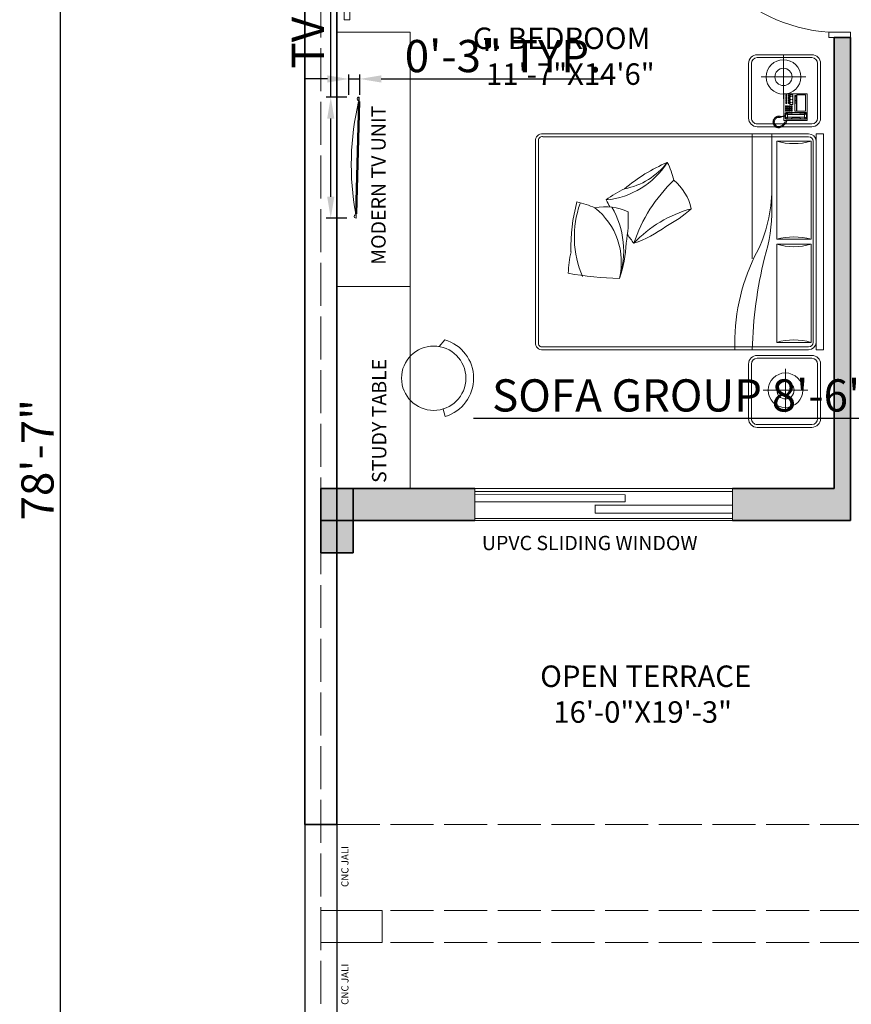
# Model space of a CAD drawing. Units: millimetres. Extents: x 595116 to 630915, y 909473 to 920225.
# Tile 129 of 134: x 630214 to 630446, y 919466 to 919741. Entities that reach past the tile are written whole.
import ezdxf

# ---------------------------------------------------------------- set-up
doc = ezdxf.new("R2010")
doc.units = ezdxf.units.MM
doc.linetypes.add('ACAD_ISO02W100', pattern=[15, 12, -3])
for name, color, linetype, lineweight in [('A-AREA-IDEN', 7, 'Continuous', 20), ('A-EQPM', 8, 'Continuous', 13), ('A-FLOR-SCRN', 31, 'Continuous', 18), ('A-FLOR-SCRN-OVHD', 31, 'ACAD_ISO02W100', 13), ('A-FURN', 32, 'Continuous', 18), ('A-WALL', 1, 'Continuous', 35), ('A-WALL-PATT', 8, 'Continuous', 13), ('C-PROP', 7, 'Continuous', 25), ('C-PROP-REF', 240, 'ACAD_ISO02W100', 13), ('Column', 6, 'Continuous', 35), ('Dimension', 3, 'Continuous', 18), ('Doors', 31, 'Continuous', 20), ('Text', 7, 'Continuous', 18), ('Windows', 33, 'Continuous', 18)]:
    doc.layers.add(name, color=color, linetype=linetype, lineweight=lineweight)
doc.styles.get("Standard").update_dxf_attribs({"font": 'arial.ttf'})
doc.dimstyles.new('ISO-25', dxfattribs={"dimtxt": 9, "dimasz": 6, "dimexe": 1.25, "dimexo": 0.625, "dimtad": 1, "dimlunit": 4, "dimtxsty": 'Standard', "dimcen": 2.5, "dimadec": 0, "dimazin": 0, "dimtfac": 1, "dimtmove": 0, "dimatfit": 3, "dimfxl": 1, "dimarcsym": 0})

# ---------------------------------------------------------------- blocks, each defined once
blk = doc.blocks.new('KWD')
for points in [[(629753.63, 919957.93), (629752.54, 919957.93), (629752.54, 919953.43), (629753.63, 919953.43)], [(629787.45, 919957.93), (629787.45, 919953.43), (629788.54, 919953.43), (629788.54, 919957.93)]]:
    blk.add_lwpolyline(points, close=True)
blk.add_lwpolyline([(629753.63, 919921.79), (629753.63, 919955.68), (629754.13, 919955.68), (629754.13, 919921.8)])
blk.add_arc((629753.64, 919955.68), 33.88, 269.99, 356.196)
blk = doc.blocks.new('A$C356F0359')
for p, q in [((0.5489, 2), (2.0492, 2)), ((0.5489, 1.9489), (0.5489, 2)), ((2.0492, 1.9489), (2.0492, 2)), ((-0.0002, 1.9201), (-0.0002, 1.5401)), ((0.0198, 1.9201), (0.0198, 1.5401)), ((0.4398, 1.9801), (0.0598, 1.9801)), ((0.4398, 1.9601), (0.0598, 1.9601)), ((0.4798, 1.5401), (0.4798, 1.9201)), ((0.4998, 1.5401), (0.4998, 1.9201)), ((2.0492, 1.9489), (0.5489, 1.9489)), ((1.998, 1.9289), (0.6001, 1.9289)), ((2.0883, 1.9201), (2.0883, 1.5401)), ((2.1083, 1.9201), (2.1083, 1.5401)), ((2.5283, 1.9801), (2.1483, 1.9801)), ((2.5283, 1.9601), (2.1483, 1.9601)), ((2.5683, 1.5401), (2.5683, 1.9201)), ((2.5883, 1.5401), (2.5883, 1.9201)), ((0.1539, 1.5681), (0.1539, 1.8777)), ((0.2725, 1.8879), (0.2702, 1.8856)), ((0.2702, 1.8856), (0.2702, 1.7279)), ((0.2725, 1.8879), (0.4531, 1.8879)), ((0.3913, 1.8753), (0.277, 1.8753)), ((0.277, 1.8753), (0.277, 1.8147)), ((0.3913, 1.8147), (0.3913, 1.8753)), ((0.4016, 1.8787), (0.4062, 1.8845)), ((0.4016, 1.7404), (0.4016, 1.8787)), ((0.4062, 1.881), (0.405, 1.8765)), ((0.405, 1.8765), (0.4153, 1.8662)), ((0.405, 1.8765), (0.405, 1.8456)), ((0.4062, 1.8845), (0.4405, 1.8845)), ((0.4108, 1.8833), (0.4062, 1.881)), ((0.4108, 1.8833), (0.4382, 1.8833)), ((0.4165, 1.8685), (0.4108, 1.8833)), ((0.4153, 1.8662), (0.4165, 1.8685)), ((0.4153, 1.8147), (0.4153, 1.8662)), ((0.4325, 1.8685), (0.4165, 1.8685)), ((0.4325, 1.8685), (0.4382, 1.8833)), ((0.4336, 1.8662), (0.4325, 1.8685)), ((0.4439, 1.8765), (0.4336, 1.8662)), ((0.4336, 1.8147), (0.4336, 1.8662)), ((0.4382, 1.8833), (0.4428, 1.881)), ((0.4405, 1.8845), (0.4462, 1.8787)), ((0.4428, 1.881), (0.4439, 1.8765)), ((0.4439, 1.8765), (0.4439, 1.8456)), ((0.4462, 1.8787), (0.4462, 1.7416)), ((0.4531, 1.8879), (0.4553, 1.8856)), ((0.4553, 1.8856), (0.4553, 1.7279)), ((0.5489, 1.8977), (0.5489, 0.0512)), ((0.5689, 1.8977), (0.5689, 0.0512)), ((2.0292, 0.0512), (2.0292, 1.8977)), ((2.0492, 0.0512), (2.0492, 1.8977)), ((2.3306, 1.5822), (2.3306, 1.8917)), ((0.277, 1.8147), (0.3913, 1.8147)), ((0.277, 1.7885), (0.277, 1.7679)), ((0.3445, 1.7885), (0.277, 1.7885)), ((0.3913, 1.8125), (0.2816, 1.8125)), ((0.2816, 1.8125), (0.2816, 1.801)), ((0.2816, 1.801), (0.3913, 1.801)), ((0.2885, 1.7862), (0.2885, 1.7827)), ((0.2919, 1.7862), (0.2885, 1.7862)), ((0.2885, 1.7827), (0.2919, 1.7827)), ((0.2907, 1.8125), (0.2907, 1.801)), ((0.2919, 1.7827), (0.2919, 1.7862)), ((0.2999, 1.8125), (0.2999, 1.801)), ((0.309, 1.8125), (0.309, 1.801)), ((0.3125, 1.7862), (0.309, 1.7862)), ((0.309, 1.7862), (0.309, 1.7827)), ((0.309, 1.7827), (0.3125, 1.7827)), ((0.3125, 1.7827), (0.3125, 1.7862)), ((0.3182, 1.8125), (0.3182, 1.801)), ((0.3273, 1.8125), (0.3273, 1.801)), ((0.333, 1.7862), (0.3296, 1.7862)), ((0.3296, 1.7862), (0.3296, 1.7827)), ((0.3296, 1.7827), (0.333, 1.7827)), ((0.333, 1.7827), (0.333, 1.7862)), ((0.3365, 1.8125), (0.3365, 1.801)), ((0.3445, 1.7679), (0.3445, 1.7885)), ((0.3548, 1.7759), (0.3548, 1.7827)), ((0.3548, 1.7827), (0.3639, 1.7827)), ((0.3639, 1.7827), (0.3639, 1.7759)), ((0.3685, 1.7827), (0.3776, 1.7827)), ((0.3685, 1.7759), (0.3685, 1.7827)), ((0.3776, 1.7827), (0.3776, 1.7759)), ((0.3822, 1.7759), (0.3822, 1.7827)), ((0.3822, 1.7827), (0.3913, 1.7827)), ((0.3913, 1.801), (0.3913, 1.8125)), ((0.3913, 1.7827), (0.3913, 1.7759)), ((0.405, 1.8456), (0.4073, 1.8399)), ((0.405, 1.7736), (0.4073, 1.7793)), ((0.4073, 1.8399), (0.4108, 1.8342)), ((0.4073, 1.7793), (0.4108, 1.785)), ((0.4108, 1.8342), (0.4119, 1.8262)), ((0.4108, 1.785), (0.4119, 1.793)), ((0.4119, 1.8262), (0.4119, 1.8147)), ((0.4119, 1.793), (0.4119, 1.8147)), ((0.4153, 1.8147), (0.4153, 1.753)), ((0.4336, 1.8147), (0.4336, 1.753)), ((0.4382, 1.8342), (0.4371, 1.8262)), ((0.4371, 1.8262), (0.4371, 1.8147)), ((0.4371, 1.793), (0.4371, 1.8147)), ((0.4382, 1.785), (0.4371, 1.793)), ((0.4416, 1.8399), (0.4382, 1.8342)), ((0.4416, 1.7793), (0.4382, 1.785)), ((0.4439, 1.8456), (0.4416, 1.8399)), ((0.4439, 1.7736), (0.4416, 1.7793)), ((0.3052, 1.7226), (0.0051, 1.7226)), ((0.2702, 1.7279), (0.2725, 1.7256)), ((0.4244, 1.7256), (0.2725, 1.7256)), ((0.277, 1.7679), (0.3445, 1.7679)), ((0.2782, 1.7622), (0.2782, 1.7576)), ((0.2896, 1.7622), (0.2782, 1.7622)), ((0.2782, 1.7576), (0.2896, 1.7576)), ((0.2782, 1.745), (0.2896, 1.745)), ((0.2782, 1.7382), (0.2782, 1.745)), ((0.2896, 1.7382), (0.2782, 1.7382)), ((0.2919, 1.7736), (0.2885, 1.7736)), ((0.2885, 1.7736), (0.2885, 1.7702)), ((0.2885, 1.7702), (0.2919, 1.7702)), ((0.2896, 1.7576), (0.2896, 1.7622)), ((0.2896, 1.745), (0.2896, 1.7382)), ((0.2919, 1.7702), (0.2919, 1.7736)), ((0.2942, 1.7622), (0.2942, 1.7576)), ((0.3056, 1.7622), (0.2942, 1.7622)), ((0.2942, 1.7576), (0.3056, 1.7576)), ((0.2942, 1.745), (0.3056, 1.745)), ((0.2942, 1.7382), (0.2942, 1.745)), ((0.3056, 1.7382), (0.2942, 1.7382)), ((0.3056, 1.7576), (0.3056, 1.7622)), ((0.3056, 1.745), (0.3056, 1.7382)), ((0.3125, 1.7736), (0.309, 1.7736)), ((0.309, 1.7736), (0.309, 1.7702)), ((0.309, 1.7702), (0.3125, 1.7702)), ((0.3102, 1.7622), (0.3102, 1.7576)), ((0.3216, 1.7622), (0.3102, 1.7622)), ((0.3102, 1.7576), (0.3216, 1.7576)), ((0.3102, 1.745), (0.3216, 1.745)), ((0.3102, 1.7382), (0.3102, 1.745)), ((0.3216, 1.7382), (0.3102, 1.7382)), ((0.3125, 1.7702), (0.3125, 1.7736)), ((0.3216, 1.7576), (0.3216, 1.7622)), ((0.3216, 1.745), (0.3216, 1.7382)), ((0.3376, 1.7622), (0.3262, 1.7622)), ((0.3262, 1.7622), (0.3262, 1.7576)), ((0.3262, 1.7576), (0.3376, 1.7576)), ((0.3262, 1.7382), (0.3262, 1.745)), ((0.3262, 1.745), (0.3376, 1.745)), ((0.3376, 1.7382), (0.3262, 1.7382)), ((0.333, 1.7736), (0.3296, 1.7736)), ((0.3296, 1.7736), (0.3296, 1.7702)), ((0.3296, 1.7702), (0.333, 1.7702)), ((0.333, 1.7702), (0.333, 1.7736)), ((0.3376, 1.7576), (0.3376, 1.7622)), ((0.3376, 1.745), (0.3376, 1.7382)), ((0.3639, 1.7759), (0.3548, 1.7759)), ((0.3548, 1.7633), (0.3548, 1.7702)), ((0.3548, 1.7702), (0.3639, 1.7702)), ((0.3639, 1.7633), (0.3548, 1.7633)), ((0.3548, 1.7564), (0.3639, 1.7564)), ((0.3548, 1.7496), (0.3548, 1.7564)), ((0.3639, 1.7496), (0.3548, 1.7496)), ((0.3548, 1.737), (0.3548, 1.7439)), ((0.3548, 1.7439), (0.3639, 1.7439)), ((0.3639, 1.737), (0.3548, 1.737)), ((0.3639, 1.7702), (0.3639, 1.7633)), ((0.3639, 1.7564), (0.3639, 1.7496)), ((0.3639, 1.7439), (0.3639, 1.737)), ((0.3776, 1.7759), (0.3685, 1.7759)), ((0.3685, 1.7633), (0.3685, 1.7702)), ((0.3685, 1.7702), (0.3776, 1.7702)), ((0.3776, 1.7633), (0.3685, 1.7633)), ((0.3685, 1.7564), (0.3776, 1.7564)), ((0.3685, 1.7496), (0.3685, 1.7564)), ((0.3776, 1.7496), (0.3685, 1.7496)), ((0.3685, 1.737), (0.3685, 1.7439)), ((0.3685, 1.7439), (0.3776, 1.7439)), ((0.3776, 1.737), (0.3685, 1.737)), ((0.3776, 1.7702), (0.3776, 1.7633)), ((0.3776, 1.7564), (0.3776, 1.7496)), ((0.3776, 1.7439), (0.3776, 1.737)), ((0.3913, 1.7759), (0.3822, 1.7759)), ((0.3822, 1.7633), (0.3822, 1.7702)), ((0.3822, 1.7702), (0.3913, 1.7702)), ((0.3913, 1.7633), (0.3822, 1.7633)), ((0.3822, 1.7576), (0.3913, 1.7576)), ((0.3822, 1.7507), (0.3822, 1.7576)), ((0.3913, 1.7507), (0.3822, 1.7507)), ((0.3822, 1.7439), (0.3913, 1.7439)), ((0.3822, 1.737), (0.3822, 1.7439)), ((0.3913, 1.737), (0.3822, 1.737)), ((0.3913, 1.7702), (0.3913, 1.7633)), ((0.3913, 1.7576), (0.3913, 1.7507)), ((0.3913, 1.7439), (0.3913, 1.737)), ((0.4073, 1.7347), (0.4016, 1.7404)), ((0.405, 1.7427), (0.405, 1.7736)), ((0.405, 1.7427), (0.4153, 1.753)), ((0.4062, 1.7382), (0.405, 1.7427)), ((0.4108, 1.7359), (0.4062, 1.7382)), ((0.4234, 1.7347), (0.4073, 1.7347)), ((0.4165, 1.7507), (0.4108, 1.7359)), ((0.4108, 1.7359), (0.4234, 1.7359)), ((0.4153, 1.753), (0.4165, 1.7507)), ((0.4325, 1.7507), (0.4165, 1.7507)), ((0.4233, 1.7393), (0.4235, 1.7294)), ((0.4268, 1.7393), (0.4233, 1.7393)), ((0.4235, 1.7294), (0.4263, 1.7179)), ((0.4263, 1.7179), (0.429, 1.707)), ((0.4274, 1.7301), (0.4268, 1.7393)), ((0.427, 1.7359), (0.4382, 1.7359)), ((0.4405, 1.7347), (0.4271, 1.7347)), ((0.429, 1.7227), (0.4274, 1.7301)), ((0.4531, 1.7256), (0.4284, 1.7256)), ((0.4318, 1.7119), (0.429, 1.7227)), ((0.4325, 1.7063), (0.4318, 1.7119)), ((0.4336, 1.753), (0.4325, 1.7507)), ((0.4325, 1.7507), (0.4382, 1.7359)), ((0.4439, 1.7427), (0.4336, 1.753)), ((0.4382, 1.7359), (0.4428, 1.7382)), ((0.4462, 1.7416), (0.4405, 1.7347)), ((0.4428, 1.7382), (0.4439, 1.7427)), ((0.4439, 1.7427), (0.4439, 1.7736)), ((0.4553, 1.7279), (0.4531, 1.7256)), ((0.4622, 1.7459), (0.4553, 1.7484)), ((0.4553, 1.7439), (0.4604, 1.7425)), ((0.4604, 1.7425), (0.465, 1.7388)), ((0.4654, 1.7427), (0.4622, 1.7459)), ((0.465, 1.7388), (0.4662, 1.7372)), ((0.4678, 1.7405), (0.4654, 1.7427)), ((0.4662, 1.7372), (0.4686, 1.7374)), ((0.4686, 1.7374), (0.4662, 1.735)), ((0.4662, 1.735), (0.4755, 1.7268)), ((0.4721, 1.7421), (0.4678, 1.7405)), ((0.4741, 1.7401), (0.4721, 1.7421)), ((0.4725, 1.7366), (0.4741, 1.7401)), ((0.4753, 1.7388), (0.4725, 1.7366)), ((0.4783, 1.7356), (0.4753, 1.7388)), ((0.4755, 1.7268), (0.4906, 1.7139)), ((0.4759, 1.729), (0.4783, 1.7356)), ((0.4821, 1.7322), (0.4759, 1.729)), ((0.4874, 1.7272), (0.4821, 1.7322)), ((0.4862, 1.7199), (0.4874, 1.7272)), ((0.4914, 1.7231), (0.4862, 1.7199)), ((0.4908, 1.7135), (0.4984, 1.6917)), ((0.4958, 1.7185), (0.4914, 1.7231)), ((0.494, 1.7135), (0.4958, 1.7185)), ((0.501, 1.7142), (0.494, 1.7135)), ((0.5031, 1.7072), (0.501, 1.7142)), ((2.4819, 1.7366), (2.1818, 1.7366)), ((0.427, 1.697), (0.4265, 1.6915)), ((0.4265, 1.6915), (0.4332, 1.6903)), ((0.4332, 1.6903), (0.4267, 1.6864)), ((0.4267, 1.6864), (0.4272, 1.6801)), ((0.4295, 1.6996), (0.427, 1.697)), ((0.4272, 1.6801), (0.4346, 1.6794)), ((0.4346, 1.6794), (0.4281, 1.6744)), ((0.4281, 1.6744), (0.4311, 1.669)), ((0.429, 1.707), (0.4288, 1.701)), ((0.4288, 1.701), (0.4295, 1.6996)), ((0.4311, 1.669), (0.4381, 1.6704)), ((0.4323, 1.7003), (0.4325, 1.7063)), ((0.4364, 1.6973), (0.4323, 1.7003)), ((0.4381, 1.6704), (0.4348, 1.6639)), ((0.4348, 1.6639), (0.4383, 1.6598)), ((0.4355, 1.6919), (0.4364, 1.6973)), ((0.4367, 1.6774), (0.4355, 1.6919)), ((0.4455, 1.6663), (0.4367, 1.6774)), ((0.4383, 1.6598), (0.4436, 1.6637)), ((0.4436, 1.6637), (0.4427, 1.6575)), ((0.4427, 1.6575), (0.4471, 1.6547)), ((0.4577, 1.6598), (0.4455, 1.6663)), ((0.4471, 1.6547), (0.4526, 1.6593)), ((0.4526, 1.6593), (0.4519, 1.6517)), ((0.4519, 1.6517), (0.4568, 1.6503)), ((0.4568, 1.6503), (0.4598, 1.6565)), ((0.4716, 1.6586), (0.4577, 1.6598)), ((0.4598, 1.6565), (0.4626, 1.6503)), ((0.4626, 1.6503), (0.4665, 1.6498)), ((0.4665, 1.6498), (0.4681, 1.6565)), ((0.4681, 1.6565), (0.4707, 1.6491)), ((0.4707, 1.6491), (0.4751, 1.6503)), ((0.485, 1.6644), (0.4716, 1.6586)), ((0.4751, 1.6503), (0.4753, 1.6565)), ((0.4753, 1.6565), (0.4806, 1.6519)), ((0.4806, 1.6519), (0.4843, 1.6538)), ((0.4843, 1.6538), (0.4836, 1.6607)), ((0.4836, 1.6607), (0.4885, 1.6547)), ((0.4952, 1.6744), (0.485, 1.6644)), ((0.4885, 1.6547), (0.4922, 1.6579)), ((0.4922, 1.6579), (0.4894, 1.6642)), ((0.4894, 1.6642), (0.4959, 1.6614)), ((0.4984, 1.6917), (0.4952, 1.6744)), ((0.4957, 1.6704), (0.5024, 1.6683)), ((0.4989, 1.6642), (0.4957, 1.6704)), ((0.4959, 1.6614), (0.4989, 1.6642)), ((0.4964, 1.7047), (0.5031, 1.7072)), ((0.5038, 1.7049), (0.4964, 1.7047)), ((0.5042, 1.673), (0.4987, 1.6792)), ((0.4987, 1.6792), (0.5058, 1.679)), ((0.5005, 1.695), (0.5054, 1.6996)), ((0.5068, 1.695), (0.5005, 1.695)), ((0.5008, 1.6871), (0.5079, 1.6892)), ((0.5068, 1.6836), (0.5008, 1.6871)), ((0.5024, 1.6683), (0.5042, 1.673)), ((0.5054, 1.6996), (0.5038, 1.7049)), ((0.5058, 1.679), (0.5068, 1.6836)), ((0.5079, 1.6892), (0.5068, 1.695)), ((0.0598, 1.5001), (0.4398, 1.5001)), ((0.0598, 1.4801), (0.4398, 1.4801)), ((2.1483, 1.5001), (2.5283, 1.5001)), ((2.1483, 1.4801), (2.5283, 1.4801)), ((0.6001, 0.02), (1.998, 0.02)), ((0.6001, 0), (1.998, 0))]:
    blk.add_line(p, q)
at = {"linetype": 'ByBlock'}
for p, q in [((0.6001, 1.9147), (1.282, 1.9147)), ((0.6001, 1.6759), (0.6001, 1.9147)), ((1.282, 1.9147), (1.282, 1.6759)), ((1.3161, 1.9147), (1.998, 1.9147)), ((1.3161, 1.6759), (1.3161, 1.9147)), ((1.998, 1.9147), (1.998, 1.6759)), ((1.282, 1.6759), (0.6001, 1.6759)), ((1.998, 1.6759), (1.3161, 1.6759)), ((1.0687, 1.6418), (0.5489, 1.6418)), ((1.4185, 1.5053), (0.5489, 1.5053))]:
    blk.add_line(p, q, dxfattribs=at)
for centre in [(2.3306, 1.7366), (0.1539, 1.7226)]:
    blk.add_circle(centre, 0.12, dxfattribs=at)
for centre in [(0.1539, 1.7226), (2.3306, 1.7366)]:
    blk.add_circle(centre, 0.06)
for centre, radius, start, end in [((0.0598, 1.9201), 0.06, 90, 180), ((0.0598, 1.9201), 0.04, 90, 180), ((0.4398, 1.9201), 0.06, 0, 90), ((0.4398, 1.9201), 0.04, 0, 90), ((0.6001, 1.8977), 0.0512, 90, 180), ((0.6001, 1.8977), 0.0312, 90, 180), ((1.998, 1.8977), 0.0512, 0, 90), ((1.998, 1.8977), 0.0312, 0, 90), ((2.1483, 1.9201), 0.06, 90, 180), ((2.1483, 1.9201), 0.04, 90, 180), ((2.5283, 1.9201), 0.06, 0, 90), ((2.5283, 1.9201), 0.04, 0, 90), ((0.0598, 1.5401), 0.06, 180, 270), ((0.0598, 1.5401), 0.04, 180, 270), ((0.4398, 1.5401), 0.04, 270, 0), ((0.4398, 1.5401), 0.06, 270, 0), ((2.1483, 1.5401), 0.06, 180, 270), ((2.1483, 1.5401), 0.04, 180, 270), ((2.5283, 1.5401), 0.06, 270, 0), ((2.5283, 1.5401), 0.04, 270, 0), ((1.1471, 0.7332), 0.3575, 102.47819, 140.46254), ((1.9086, 1.3124), 0.8697, 195.33601, 226.41927), ((0.3249, 0.4335), 0.9879, 28.49711, 41.05657), ((0.9965, 0.4273), 0.548, 103.20343, 117.03623), ((1.6529, 1.7059), 1.0798, 223.63057, 251.4288), ((0.4451, 0.4375), 0.5655, 5.33912, 57.68949), ((0.4517, 0.5274), 0.4879, 10.69865, 52.68638), ((1.8195, 1.3719), 1.1652, 203.06416, 220.32086), ((0.5617, 0.4344), 0.7874, 18.35266, 36.68512), ((1.5949, 0.9312), 0.734, 205.25901, 216.93514), ((1.4135, 0.487), 0.3575, 154.0418, 192.02615), ((1.1372, -0.3434), 0.9879, 80.06073, 92.62018), ((-0.021, 2.4319), 2.1977, 305.29657, 307.24182), ((1.2836, -0.1573), 0.7874, 69.91627, 88.24873), ((1.3641, 0.0041), 0.6085, 71.81005, 120.13512), ((1.44, 0.1186), 0.4774, 76.18494, 142.00166), ((-0.6432, 0.628), 2.1977, 349.48843, 358.80544), ((-0.021, 2.4319), 2.1977, 297.92482, 299.3793), ((1.5595, 0.1789), 0.548, 154.76704, 168.59984), ((1.3312, 1.4107), 1.1652, 254.62778, 271.88448), ((1.2647, 0.9578), 0.6885, 250.29361, 293.6414), ((1.5368, 0.9609), 0.734, 256.82263, 268.49876), ((0.5943, 0.0454), 0.0458, 172.75992, 277.24008), ((0.5943, 0.0454), 0.0258, 172.75992, 277.24008), ((2.0038, 0.0454), 0.0458, 262.75992, 7.24008), ((2.0038, 0.0454), 0.0258, 262.75992, 7.24008)]:
    blk.add_arc(centre, radius, start, end)
for centre, radius, start, end in [((0.1906, 1.7953), 0.4265, 343.73979, 16.26021), ((1.6914, 1.7953), 0.4265, 163.73979, 196.26021), ((0.9067, 1.7953), 0.4265, 343.73979, 16.26021), ((2.4075, 1.7953), 0.4265, 163.73979, 196.26021), ((1.0826, 0.5712), 1.0706, 72.19663, 90.74184), ((0.9303, 0.657), 0.9853, 61.43285, 88.12613), ((2.1368, 4.5996), 3.0955, 256.42012, 268.37887), ((2.0056, 2.7745), 1.3903, 244.24266, 271.79845)]:
    blk.add_arc(centre, radius, start, end, dxfattribs=at)
blk = doc.blocks.new('TV-SCREEN')
for p, q in [((2.14, 32.58), (2.14, 33.76)), ((2.19, 32.58), (2.19, 33.76)), ((2.04, 32.58), (1.21, 1.19)), ((2.14, 32.58), (1.31, 1.19)), ((2.24, 32.58), (1.41, 1.19)), ((2.34, 32.57), (1.51, 1.18)), ((1.31, 1.19), (1.31, 0.01)), ((1.36, 1.19), (1.36, 0.01))]:
    blk.add_line(p, q)
for centre, radius, start, end in [((2.09, 33.31), 0.462, 77.1755, 282.8245), ((76.63, 14.9), 76.65, 166.662, 190.3006), ((1.26, 0.46), 0.462, 77.1755, 282.8245)]:
    blk.add_arc(centre, radius, start, end)
blk = doc.blocks.new('CHAIR-ROUND-2')
for p, q in [((12.11, 21.41), (10.53, 19.55)), ((12.22, 0), (11.59, 2.08))]:
    blk.add_line(p, q)
blk.add_circle((8.99, 10.69), 8.99)
blk.add_arc((8.99, 10.69), 11.16, 286.7943, 73.7898)
blk = doc.blocks.new('COLUMN-RECT-9X18')
h = blk.add_hatch(color=256)
h.dxf.hatch_style = 1
h.paths.add_polyline_path([(9, 18), (0, 18), (0, 0), (9, 0)])
blk.add_lwpolyline([(0, 18), (9, 18), (9, 0), (0, 0)], close=True)
blk = doc.blocks.new('*D176')
at = {"layer": 'Defpoints', "color": 0, "transparency": 16777216}
for p in [(630300.87, 919719.25), (630305.94, 919719.25), (630305.94, 919685.42)]:
    blk.add_point(p, dxfattribs=at)
at = {"layer": 'Dimension', "color": 0, "lineweight": -2, "transparency": 16777216}
for p, q in [((630300.87, 919719.25), (630300.87, 919808.14)), ((630305.32, 919719.25), (630299.62, 919719.25)), ((630300.87, 919691.42), (630300.87, 919713.25)), ((630305.32, 919685.42), (630299.62, 919685.42))]:
    blk.add_line(p, q, dxfattribs=at)
at = {"layer": 'Dimension', "color": 0, "transparency": 16777216}
for points in [[(630299.87, 919713.25), (630301.87, 919713.25), (630300.87, 919719.25)], [(630299.87, 919691.42), (630301.87, 919691.42), (630300.87, 919685.42)]]:
    blk.add_solid(points, dxfattribs=at)
at = {"layer": 'Dimension', "color": 0, "transparency": 16777216, "insert": (630295.65, 919766.69), "char_height": 9, "attachment_point": 5, "rotation": 90}
blk.add_mtext('TV 2\'-10" TYP.', dxfattribs=at)
blk = doc.blocks.new('*D177')
at = {"layer": 'Defpoints', "color": 0, "transparency": 16777216}
for p in [(630308.97, 919724.32), (630305.94, 919719.25), (630308.97, 919719.25)]:
    blk.add_point(p, dxfattribs=at)
at = {"layer": 'Dimension', "color": 0, "lineweight": -2, "transparency": 16777216}
for p, q in [((630299.94, 919724.32), (630293.94, 919724.32)), ((630305.94, 919719.87), (630305.94, 919725.57)), ((630305.94, 919724.32), (630308.97, 919724.32)), ((630308.97, 919719.87), (630308.97, 919725.57)), ((630314.97, 919724.32), (630377.08, 919724.32))]:
    blk.add_line(p, q, dxfattribs=at)
at = {"layer": 'Dimension', "color": 0, "transparency": 16777216}
for points in [[(630299.94, 919725.32), (630299.94, 919723.32), (630305.94, 919724.32)], [(630314.97, 919725.32), (630314.97, 919723.32), (630308.97, 919724.32)]]:
    blk.add_solid(points, dxfattribs=at)
at = {"layer": 'Dimension', "color": 0, "transparency": 16777216, "insert": (630349.02, 919729.55), "char_height": 9, "attachment_point": 5}
blk.add_mtext('0\'-3" TYP.', dxfattribs=at)
blk = doc.blocks.new('*D182')
at = {"layer": 'Defpoints', "color": 0, "transparency": 16777216}
for p in [(630490.2, 919644.73), (630592.04, 919644.73), (630490.2, 919629.46)]:
    blk.add_point(p, dxfattribs=at)
at = {"layer": 'Dimension', "color": 0, "lineweight": -2, "transparency": 16777216}
for p, q in [((630490.2, 919644.11), (630490.2, 919628.21)), ((630592.04, 919644.11), (630592.04, 919628.21)), ((630490.2, 919629.46), (630340.81, 919629.46)), ((630586.04, 919629.46), (630496.2, 919629.46))]:
    blk.add_line(p, q, dxfattribs=at)
at = {"layer": 'Dimension', "color": 0, "transparency": 16777216}
for points in [[(630496.2, 919630.46), (630496.2, 919628.46), (630490.2, 919629.46)], [(630586.04, 919630.46), (630586.04, 919628.46), (630592.04, 919629.46)]]:
    blk.add_solid(points, dxfattribs=at)
at = {"layer": 'Dimension', "color": 0, "transparency": 16777216, "insert": (630412.5, 919634.74), "char_height": 9, "attachment_point": 5}
blk.add_mtext('SOFA GROUP 8\'-6" TYP.', dxfattribs=at)
blk = doc.blocks.new('*D214')
at = {"layer": 'Defpoints', "color": 0, "transparency": 16777216}
for p in [(630293.6, 920089.43), (630225.3, 919146.43), (630293.6, 919146.43)]:
    blk.add_point(p, dxfattribs=at)
at = {"layer": 'Dimension', "color": 0, "lineweight": -2, "transparency": 16777216}
for p, q in [((630292.97, 920089.43), (630224.05, 920089.43)), ((630225.3, 920083.43), (630225.3, 919152.43)), ((630292.97, 919146.43), (630224.05, 919146.43))]:
    blk.add_line(p, q, dxfattribs=at)
at = {"layer": 'Dimension', "color": 0, "transparency": 16777216}
for points in [[(630224.3, 920083.43), (630226.3, 920083.43), (630225.3, 920089.43)], [(630224.3, 919152.43), (630226.3, 919152.43), (630225.3, 919146.43)]]:
    blk.add_solid(points, dxfattribs=at)
at = {"layer": 'Dimension', "color": 0, "transparency": 16777216, "insert": (630220.08, 919617.93), "char_height": 9, "attachment_point": 5, "rotation": 90}
blk.add_mtext('78\'-7"', dxfattribs=at)

msp = doc.modelspace()

# ---------------------------------------------------------------- hatches: boundary and pattern name
at = {"layer": 'A-WALL-PATT'}
h = msp.add_hatch(color=256, dxfattribs=at)
h.dxf.hatch_style = 1
h.paths.add_polyline_path([(630446.096, 919735.928), (630441.596, 919735.928), (630441.596, 919609.928), (630413.111, 919609.928), (630413.111, 919600.928), (630446.096, 919600.928)])
h = msp.add_hatch(color=256, dxfattribs=at)
h.dxf.hatch_style = 1
h.paths.add_polyline_path([(630341.111, 919609.928), (630307.096, 919609.928), (630307.096, 919600.928), (630341.111, 919600.928)])

# ---------------------------------------------------------------- linework, layer by layer
at = {"layer": 'A-FLOR-SCRN'}
msp.add_lwpolyline([(630298.096, 919492.015), (630315.223, 919492.015), (630315.223, 919483.015), (630298.096, 919483.015)], close=True, dxfattribs=at)
at = {"layer": 'A-FLOR-SCRN-OVHD'}
for p, q in [((630302.596, 919516.015), (630494.596, 919516.015)), ((630302.596, 919492.015), (630494.596, 919492.015)), ((630302.596, 919483.015), (630494.596, 919483.015))]:
    msp.add_line(p, q, dxfattribs=at)
at = {"layer": 'A-FURN'}
for p, q in [((630323.082, 919737.428), (630302.596, 919737.428)), ((630323.082, 919737.428), (630323.082, 919609.928)), ((630302.596, 919666.294), (630323.082, 919666.294))]:
    msp.add_line(p, q, dxfattribs=at)
msp.add_lwpolyline([(630306.233, 919785.867), (630304.64, 919785.867), (630304.64, 919740.848), (630306.233, 919740.848)], close=True, dxfattribs=at)
at = {"layer": 'A-WALL'}
for p, q in [((630302.596, 919516.015), (630302.596, 920022.301)), ((630441.596, 919609.928), (630441.596, 919735.928)), ((630441.596, 919735.928), (630446.096, 919735.928)), ((630446.096, 919600.928), (630446.096, 919735.928)), ((630298.096, 919609.928), (630341.111, 919609.928)), ((630413.111, 919609.928), (630441.596, 919609.928)), ((630298.096, 919600.928), (630341.111, 919600.928)), ((630413.111, 919600.928), (630446.096, 919600.928)), ((630293.596, 919516.015), (630302.596, 919516.015))]:
    msp.add_line(p, q, dxfattribs=at)
msp.add_lwpolyline([(630293.596, 919516.015), (630293.596, 920022.301)], dxfattribs=at)
at = {"layer": 'C-PROP'}
for p, q in [((630293.596, 919516.015), (630293.596, 919146.428)), ((630302.596, 919516.015), (630302.596, 919429.828))]:
    msp.add_line(p, q, dxfattribs=at)
at = {"layer": 'C-PROP-REF'}
msp.add_line((630298.096, 919150.928), (630298.096, 920084.928), dxfattribs=at)
at = {"layer": 'Windows'}
for p, q in [((630341.111, 919609.928), (630341.111, 919600.928)), ((630341.111, 919609.928), (630413.111, 919609.928)), ((630413.111, 919609.928), (630413.111, 919600.928)), ((630341.113, 919606.211), (630383.111, 919606.126)), ((630341.117, 919608.211), (630383.111, 919608.126)), ((630383.111, 919608.126), (630383.107, 919606.126)), ((630413.111, 919605.26), (630374.714, 919605.26)), ((630374.756, 919603.013), (630374.756, 919605.26)), ((630341.111, 919600.928), (630413.111, 919600.928)), ((630413.111, 919603.013), (630374.756, 919603.013))]:
    msp.add_line(p, q, dxfattribs=at)
msp.add_lwpolyline([(630341.111, 919609.023), (630413.111, 919609.023), (630413.111, 919601.497), (630341.111, 919601.497)], close=True, dxfattribs=at)

# ---------------------------------------------------------------- block references
at = {"layer": 'A-EQPM'}
msp.add_blockref('TV-SCREEN', (630306.623, 919685.448), dxfattribs=at)
at = {"layer": 'A-FURN', "xscale": 40.21338437233606, "yscale": 40.21338437233606, "zscale": 40.21338437233606, "rotation": 270}
msp.add_blockref('A$C356F0359', (630358.113, 919731.069), dxfattribs=at)
at = {"layer": 'A-FURN'}
msp.add_blockref('CHAIR-ROUND-2', (630320.654, 919630.023), dxfattribs=at)
at = {"layer": 'Column'}
msp.add_blockref('COLUMN-RECT-9X18', (630298.096, 919591.928), dxfattribs=at)
at = {"layer": 'Doors', "xscale": 1.333333333333333, "yscale": 1.333333333333333, "zscale": 1.333333333333333, "rotation": 270}
msp.add_blockref('KWD', (-596164.474, 1759453.982), dxfattribs=at)

# ---------------------------------------------------------------- texts
at = {"layer": 'A-AREA-IDEN', "char_height": 6, "attachment_point": 1}
for s, insert in [('{G. BEDROOM\\P  11\'-7"X14\'6"}', (630340.621, 919738.679)), ('{OPEN TERRACE\\P  16\'-0"X19\'-3"}', (630359.401, 919560.446))]:
    msp.add_mtext_dynamic_manual_height_columns(s, width=83.57324, gutter_width=12.5, heights=[0], dxfattribs=dict(at, insert=insert))
at = {"layer": 'Text', "attachment_point": 1, "rotation": 90}
for s, width, insert, char_height in [('{     MODERN TV UNIT}', 72.55106, (630312.208, 919666.294), 4), ('{     STUDY TABLE}', 72.55106, (630312.395, 919605.351), 4), ('{CNC JALI}', 125.26422, (630303.831, 919498.556), 2), ('{CNC JALI}', 125.26422, (630303.831, 919465.641), 2)]:
    msp.add_mtext_dynamic_manual_height_columns(s, width=width, gutter_width=12.5, heights=[0], dxfattribs=dict(at, insert=insert, char_height=char_height))
at = {"layer": 'Text', "insert": (630341.894, 919596.673), "char_height": 4, "attachment_point": 1}
msp.add_mtext_dynamic_manual_height_columns('{ UPVC SLIDING WINDOW}', width=72.55106, gutter_width=12.5, heights=[0], dxfattribs=at)

# ---------------------------------------------------------------- dimensions: what is measured, and where the dimension line sits
at = {"layer": 'Dimension'}
dim = msp.add_linear_dim(base=(630225.296, 919146.428), p1=(630293.596, 920089.428), p2=(630293.596, 919146.428), angle=90, dimstyle='ISO-25', override={"dimdec": 1, "dimlfac": 1, "dimrnd": 0, "dimzin": 1, "dimdsep": 46, "dimlunit": 4, "dimfrac": 2}, dxfattribs=at)
dim.commit()
dim.dimension.update_dxf_attribs({"geometry": '*D214', "text_midpoint": (630220.076, 919617.928)})
for base, p1, p2, angle, text, picture, middle in [((630300.869, 919719.247), (630305.943, 919685.416), (630305.943, 919719.247), 90, 'TV <> TYP.', '*D176', (630295.649, 919766.692)), ((630490.198, 919629.458), (630592.035, 919644.733), (630490.198, 919644.733), 180, 'SOFA GROUP <> TYP.', '*D182', (630412.503, 919634.739))]:
    dim = msp.add_linear_dim(base=base, p1=p1, p2=p2, angle=angle, text=text, dimstyle='ISO-25', override={"dimdec": 1, "dimlfac": 1, "dimrnd": 0, "dimzin": 1, "dimdsep": 46, "dimlunit": 4, "dimfrac": 2}, dxfattribs=at)
    dim.commit()
    dim.dimension.update_dxf_attribs({"geometry": picture, "text_midpoint": middle})
dim = msp.add_linear_dim(base=(630308.967, 919724.322), p1=(630305.943, 919719.247), p2=(630308.967, 919719.247), text='<> TYP.', dimstyle='ISO-25', override={"dimdec": 1, "dimlfac": 1, "dimrnd": 0, "dimzin": 1, "dimdsep": 46, "dimlunit": 4, "dimfrac": 2}, dxfattribs=at)
dim.commit()
dim.dimension.update_dxf_attribs({"geometry": '*D177', "text_midpoint": (630349.022, 919729.545)})

doc.saveas('drawing.dxf')
